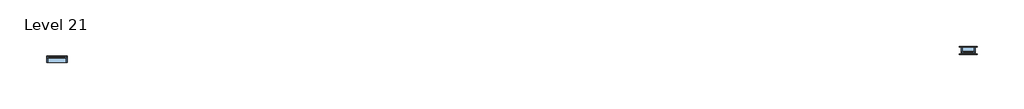
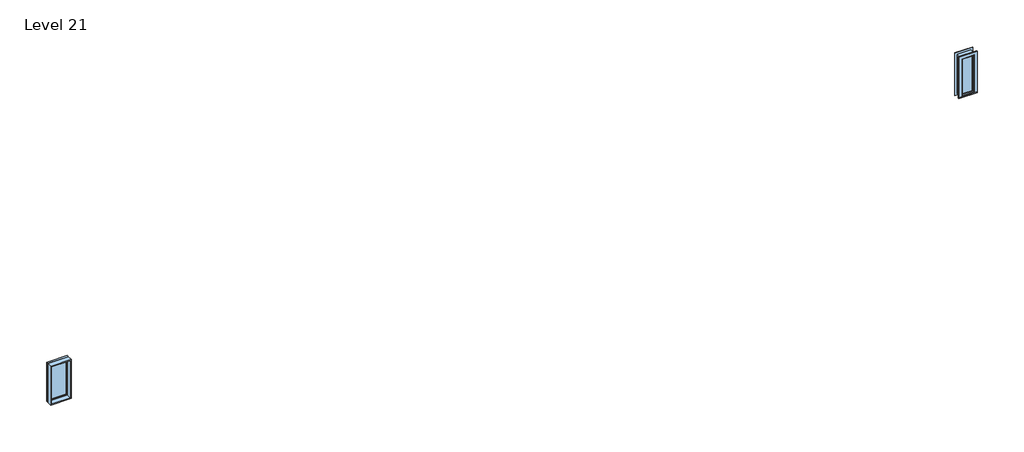
# One storey: 2 windows.
"""IFC4 building model written with IfcOpenShell, lengths in millimetres."""

from ifc_helpers import new_model, si_unit, origin, place, context, project, spatial, transform, mapped, element, save
from components import window_a765b88f, window_80bd9af0

model = new_model("IFC4")

# Units and contexts
model_context = context("Model", 3, world=origin())
ifc_project = project(units=[si_unit("LENGTHUNIT", "METRE", prefix="MILLI")], contexts=[model_context])

# Site, building, storey
site = spatial("IfcSite", under=ifc_project)
building = spatial("IfcBuilding", under=site)
storey = spatial("IfcBuildingStorey", under=building, Name="Level 21", Elevation=36271.2)

# Windows
placement = place(None, origin())
window_shape = window_a765b88f(model_context)
element("IfcWindow", 1, ObjectType="Awning with Trim : 16\" x 48\"", at=placement, inside=storey, context=model_context, shape_type="MappedRepresentation", body=[
    mapped(window_shape, transform((20663.814721, -12354.7237084, 36271.2), x_axis=(-1.0, 0.0, 0.0), y_axis=(0.0, -1.0, 0.0), z_axis=(0.0, 0.0, 1.0))),
])
window_2_shape = window_80bd9af0(model_context)
element("IfcWindow", 2, ObjectType="Fixed : 24\" x 48\"", at=placement, inside=storey, context=model_context, shape_type="MappedRepresentation", body=[
    mapped(window_2_shape, transform((-6272.885279, -12617.2007309, 36271.2), x_axis=(1.0, 0.0, 0.0), y_axis=(0.0, 1.0, 0.0), z_axis=(0.0, 0.0, 1.0))),
])

save(model, "model.ifc")

# Revit data of these elements
# Type "Awning with Trim : 16\" x 48\""
#   Type Mark = "14"
#   Construction Type Id = "GSP4R"
#   Assembly Code = "B2020100"
#   Analytic Construction = "1/8 in Pilkington single glazing"
#   Visual Light Transmittance = 0.9
#   Solar Heat Gain Coefficient = 0.78
#   Heat Transfer Coefficient (U) = 0.6496 BTU/(h·ft²·°F)
#   Height = 4' - 0"
#   Default Sill Height = 3' - 0"
#   Trim Projection - Ext. = 0' - 0 1/2"
#   Trim Projection - Int. = 0' - 0 3/4"
#   Trim Width - Exterior = 0' - 3 1/2"
#   Trim Width - Interior = 0' - 3 1/2"
#   Width = 1' - 4"
#   Window Inset = 0' - 0 3/4"
#   Define Thermal Properties by = 1
#   Glass Pane Material = Glass
#   Sash Material = Sash
#   Trim Exterior Material = Trim
#   Trim Interior Material = Trim
#   Wall Closure = (empty or 0)
# Type "Fixed : 24\" x 48\""
#   Type Mark = "2"
#   Construction Type Id = "GSP4R"
#   Assembly Code = "B2020100"
#   Analytic Construction = "1/8 in Pilkington single glazing"
#   Visual Light Transmittance = 0.9
#   Solar Heat Gain Coefficient = 0.78
#   Heat Transfer Coefficient (U) = 0.6496 BTU/(h·ft²·°F)
#   Height = 4' - 0"
#   Default Sill Height = 3' - 0"
#   Width = 2' - 0"
#   Window Inset = 0' - 0 3/4"
#   Define Thermal Properties by = 1
#   Glass Pane Material = Glass
#   Sash Material = Sash
#   Wall Closure = (empty or 0)
# Element 1 (IfcWindow, "Awning with Trim : 16\" x 48\"")
#   Mark = "57"
#   Phase Created = New Construction
#   Materials on its faces: "Sash", "Trim", "Glass"
# Element 2 (IfcWindow, "Fixed : 24\" x 48\"")
#   Mark = "74"
#   Phase Created = New Construction
#   Materials on its faces: "Sash", "Glass"
# Materials
#   "Glass": class "Glass", colour RGB 0 128 192, transparency 0.75, Description = "Soda Lime Glass", Cost = 0
#   "Sash": class "Wood", colour RGB 224 178 126, transparency 0
#   "Trim": class "Wood", colour RGB 224 178 126, transparency 0
